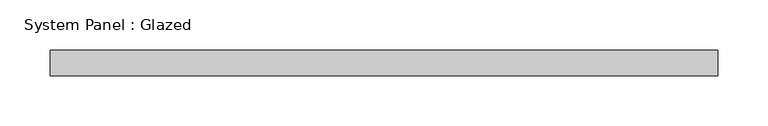
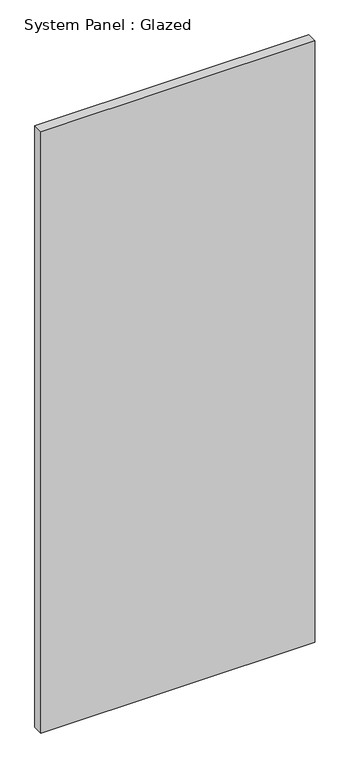
"""IFC4 building model written with IfcOpenShell, lengths in millimetres: plate geometry, System Panel : Glazed."""

from ifc_helpers import new_model, si_unit, origin, origin_with_axes, place, context, project, spatial, polyline, outline, extrude, source, transform, mapped, element, save


def system_panel_glazed_31f7001e(model_context):
    return source(origin(), model_context, "Body", "SweptSolid", [
        extrude(outline(polyline([(333.375, 19.05), (-333.375, 19.05), (-333.375, 44.45), (333.375, 44.45), (333.375, 19.05)])), origin_with_axes(), (0.0, 0.0, 1.0), 1549.4),
    ])


if __name__ == "__main__":
    model = new_model("IFC4")
    model_context = context("Model", 3, world=origin())
    ifc_project = project(units=[si_unit("LENGTHUNIT", "METRE", prefix="MILLI")], contexts=[model_context])
    site = spatial("IfcSite", under=ifc_project)
    building = spatial("IfcBuilding", under=site)
    placement = place(None, origin())
    system_panel_glazed_shape = system_panel_glazed_31f7001e(model_context)
    element("IfcPlate", 1, ObjectType="System Panel : Glazed", at=placement, inside=building, context=model_context, shape_type="MappedRepresentation", body=[
        mapped(system_panel_glazed_shape, transform((0.0, 0.0, 0.0), x_axis=(1.0, 0.0, 0.0), y_axis=(0.0, 1.0, 0.0), z_axis=(0.0, 0.0, 1.0))),
    ])
    save(model, "model.ifc")

# Revit data of these elements
# Type "System Panel : Glazed"
#   Construction Type Id = "GSP4R"
#   Analytic Construction = "1/8 in Pilkington single glazing"
#   Visual Light Transmittance = 0.9
#   Solar Heat Gain Coefficient = 0.86
#   Heat Transfer Coefficient (U) = 1.18115 BTU/(h·ft²·°F)
#   Define Thermal Properties by = 1
# Element 1 (IfcPlate, "System Panel : Glazed")
#   Materials on its faces: "Glass"
# Materials
#   "Glass": class "Glass", colour RGB 0 128 192, transparency 0.75, Description = "Soda Lime Glass", Cost = 0
